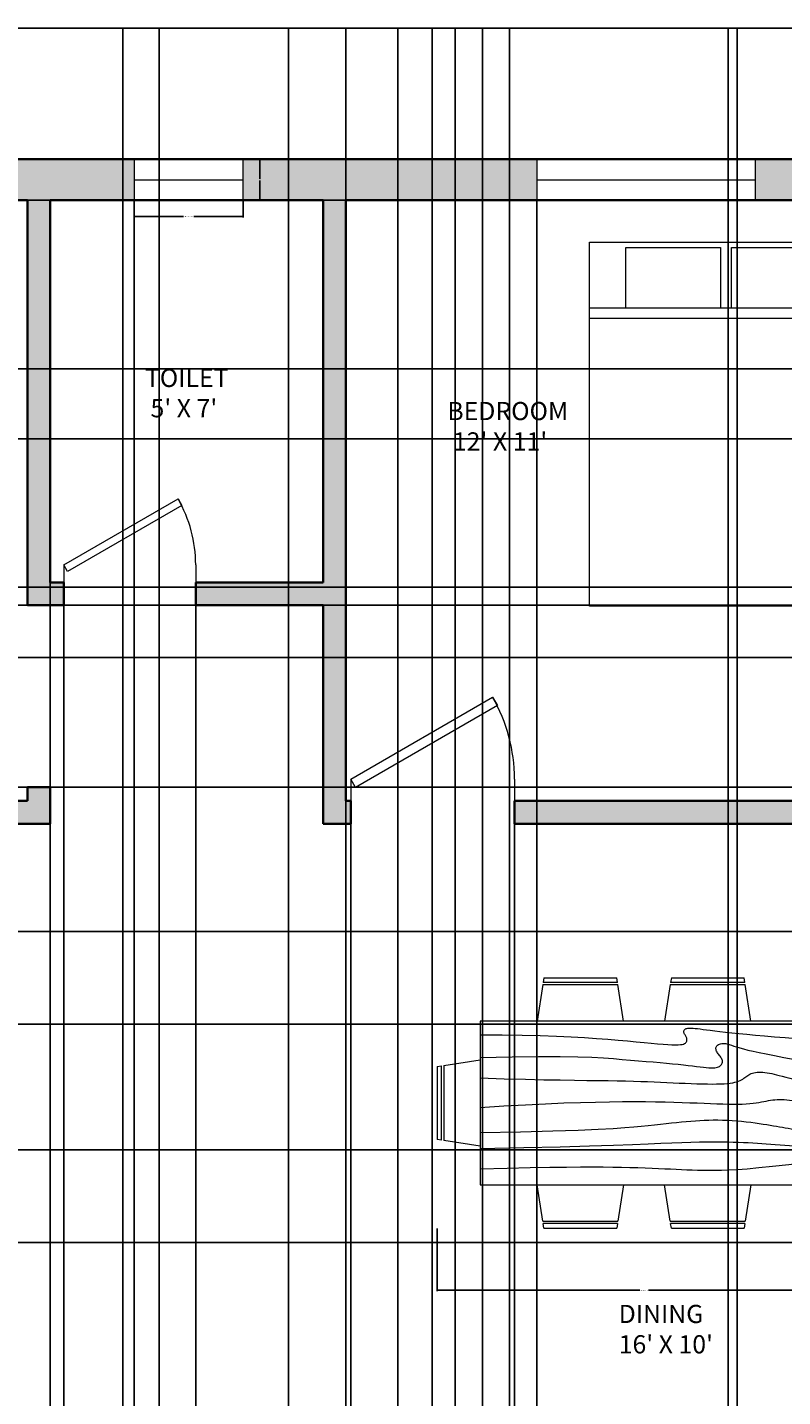
# Model space of a CAD drawing. Units: inches. Extents: x -28 to 649, y -11 to 509.
# Tile 4 of 7: x 180 to 346, y 208 to 509. Entities that reach past the tile are written whole.
import ezdxf

# ---------------------------------------------------------------- set-up
doc = ezdxf.new("R2010")
doc.units = ezdxf.units.IN
doc.header["$MEASUREMENT"] = 0
for name, color, linetype, lineweight in [('A-ANNO-DIMS', 2, 'Continuous', 18), ('A-AREA-IDEN', 18, 'Continuous', 18), ('A-WALL', 7, 'Continuous', 35), ('A-WALL-PATT', 251, 'Continuous', 13), ('doors', 40, 'Continuous', 20), ('furniture', 220, 'Continuous', 18), ('window', 30, 'Continuous', 18)]:
    doc.layers.add(name, color=color, linetype=linetype, lineweight=lineweight)
doc.styles.get("Standard").update_dxf_attribs({"font": 'arial.ttf'})
doc.dimstyles.get("Standard").update_dxf_attribs({"dimtxt": 0.18, "dimasz": 0.18, "dimexe": 0.18, "dimexo": 0.0625, "dimgap": 0.09, "dimtad": 0, "dimtih": 1, "dimtoh": 1, "dimdec": 4, "dimzin": 0, "dimdsep": 46, "dimtxsty": 'Standard', "dimcen": 0.09, "dimadec": 0, "dimazin": 0, "dimtfac": 1, "dimtdec": 4, "dimtofl": 0, "dimtmove": 0, "dimatfit": 3, "dimfxl": 1, "dimtolj": 1, "dimtzin": 0, "dimarcsym": 0})

# ---------------------------------------------------------------- blocks, each defined once
blk = doc.blocks.new('*U9')
for p, q in [((0, 0), (0, -100)), ((750, 0), (750, -100))]:
    blk.add_line(p, q)
blk.add_lwpolyline([(0, 0), (649.5, 375), (671.4, 337.1), (21.9, -37.9)], close=True)
blk.add_arc((0, 0), 750, 0, 30)
blk = doc.blocks.new('Dining Set - 36 x 72 in.')
for p, q in [((-22, 27.5), (-22.1562, 26.50042)), ((-22, 27.5), (-6, 27.5)), ((-5.8437, 26.49966), (-6, 27.5)), ((6, 27.5), (5.8438, 26.50042)), ((6, 27.5), (22, 27.5)), ((22.1563, 26.49966), (22, 27.5)), ((-22.2343, 26.00059), (-23.4847, 17.99762)), ((-22.2304, 26), (-5.7608, 26)), ((-5.8416, 26.5), (-22.1534, 26.5)), ((-4.5152, 17.99762), (-5.7655, 25.99926)), ((5.7657, 26.00059), (4.5153, 17.99762)), ((5.7696, 26), (22.2392, 26)), ((22.1584, 26.5), (5.8466, 26.5)), ((23.4848, 17.99762), (22.2345, 25.99926)), ((36, 18), (-36, 18)), ((-36, 18), (-36, -18)), ((36, -18), (36, 18)), ((-44.0006, 8.23428), (-35.9976, 9.48474)), ((44.0006, 8.23428), (35.9976, 9.48474)), ((-45.5, 8), (-44.5004, 8.15617)), ((-45.5, 8), (-45.5, -8)), ((-44.5, -8.15843), (-44.5, 8.15338)), ((-44, 8.23041), (-44, -8.23915)), ((44, 8.23041), (44, -8.23915)), ((44.5, -8.15843), (44.5, 8.15338)), ((45.5, 8), (44.5005, 8.15617)), ((45.5, 8), (45.5, -8)), ((-44.4997, -8.15631), (-45.5, -8)), ((-35.9976, -9.48476), (-43.9993, -8.2345)), ((35.9976, -9.48476), (43.9993, -8.2345)), ((44.4997, -8.15631), (45.5, -8)), ((-36, -18), (36, -18)), ((-22.2343, -26.0006), (-23.4847, -17.99762)), ((-4.5152, -17.99762), (-5.7655, -25.99928)), ((5.7657, -26.0006), (4.5153, -17.99762)), ((23.4848, -17.99762), (22.2345, -25.99928)), ((-22.2304, -26), (-5.7608, -26)), ((-22, -27.5), (-22.1562, -26.50044)), ((-5.8416, -26.5), (-22.1534, -26.5)), ((-5.8437, -26.49967), (-6, -27.5)), ((5.7696, -26), (22.2392, -26)), ((6, -27.5), (5.8438, -26.50044)), ((22.1584, -26.5), (5.8466, -26.5)), ((22.1563, -26.49967), (22, -27.5)), ((-22, -27.5), (-6, -27.5)), ((6, -27.5), (22, -27.5))]:
    blk.add_line(p, q)
for points in [[(-36, 15), (-31.1772, 14.97754), (-26.8079, 14.91406), (-22.8538, 14.81543), (-19.276, 14.6875), (-16.0362, 14.53613), (-13.0957, 14.36718), (-10.4159, 14.18652), (-7.9583, 14), (-5.6904, 13.81315), (-3.6035, 13.63021), (-1.6954, 13.45508), (0.0365, 13.29166), (1.5945, 13.14388), (2.9811, 13.01562), (4.1988, 12.9108), (5.25, 12.83333), (6.1393, 12.78613), (6.8802, 12.76823), (7.4883, 12.77767), (7.9792, 12.8125), (8.3685, 12.87077), (8.6719, 12.95052), (8.9049, 13.0498), (9.0833, 13.16666), (9.2205, 13.29899), (9.3216, 13.44401), (9.3895, 13.59879), (9.4271, 13.76041), (9.4373, 13.92594), (9.4232, 14.09245), (9.3875, 14.257), (9.3333, 14.41666), (9.2638, 14.56917), (9.1836, 14.71484), (9.0975, 14.85465), (9.0104, 14.98958), (8.9272, 15.1206), (8.8529, 15.2487), (8.7922, 15.37483), (8.75, 15.5), (8.7305, 15.62467), (8.7344, 15.74739), (8.7617, 15.86621), (8.8125, 15.97916), (8.8867, 16.08431), (8.9844, 16.17968), (9.1055, 16.26334), (9.25, 16.33333), (9.4189, 16.38802), (9.6172, 16.42708), (9.8506, 16.45052), (10.125, 16.45833), (10.4463, 16.45052), (10.8203, 16.42708), (11.2529, 16.38802), (11.75, 16.33333), (12.3184, 16.26318), (12.9694, 16.17838), (13.7151, 16.07991), (14.5677, 15.96875), (15.5395, 15.84586), (16.6426, 15.71224), (17.8893, 15.56884), (19.2917, 15.41666), (20.859, 15.25667), (22.5879, 15.08984), (24.4721, 14.91715), (26.5052, 14.73958), (28.6809, 14.5581), (30.9929, 14.3737), (33.4347, 14.18733), (36, 14)], [(-36, 10), (-28.9766, 10.14274), (-23.1725, 10.20442), (-18.4241, 10.19775), (-14.5677, 10.13541), (-11.4399, 10.03011), (-8.877, 9.89453), (-6.7154, 9.74137), (-4.7917, 9.58333), (-2.9698, 9.43082), (-1.2246, 9.28515), (0.4415, 9.14534), (2.026, 9.01041), (3.5266, 8.87939), (4.9408, 8.7513), (6.266, 8.62516), (7.5, 8.5), (8.6411, 8.37549), (9.6914, 8.2539), (10.6538, 8.13818), (11.5312, 8.03125), (12.3267, 7.93603), (13.043, 7.85547), (13.6831, 7.79248), (14.25, 7.75), (14.7471, 7.7303), (15.1797, 7.73307), (15.5537, 7.75732), (15.875, 7.80208), (16.1494, 7.86637), (16.3828, 7.94922), (16.5811, 8.04964), (16.75, 8.16666), (16.8944, 8.29915), (17.0143, 8.44531), (17.1089, 8.60319), (17.1771, 8.77083), (17.218, 8.94629), (17.2305, 9.1276), (17.2137, 9.31282), (17.1667, 9.5), (17.0895, 9.6875), (16.987, 9.875), (16.8649, 10.0625), (16.7292, 10.25), (16.5856, 10.4375), (16.4401, 10.625), (16.2985, 10.8125), (16.1667, 11), (16.05, 11.18733), (15.9518, 11.3737), (15.8752, 11.5581), (15.8229, 11.73958), (15.798, 11.91715), (15.8034, 12.08984), (15.842, 12.25667), (15.9167, 12.41666), (16.0295, 12.56836), (16.1784, 12.70833), (16.3605, 12.83268), (16.5729, 12.9375), (16.8127, 13.01888), (17.0768, 13.07291), (17.3625, 13.0957), (17.6667, 13.08333), (17.9894, 13.03312), (18.3418, 12.94726), (18.7382, 12.82918), (19.1927, 12.68229), (19.7195, 12.51001), (20.3327, 12.31575), (21.0465, 12.10294), (21.875, 11.875), (22.8357, 11.63354), (23.959, 11.37304), (25.2786, 11.08618), (26.8282, 10.76562), (28.6414, 10.40405), (30.752, 9.99414), (33.1936, 9.52856), (36, 9)], [(-36, 5.5), (-30.7157, 5.3348), (-26.069, 5.20963), (-21.9946, 5.11767), (-18.4271, 5.05208), (-15.3009, 5.00602), (-12.5508, 4.97265), (-10.1112, 4.94515), (-7.9167, 4.91666), (-5.909, 4.88167), (-4.0586, 4.83984), (-2.3429, 4.79215), (-0.7396, 4.73958), (0.7739, 4.6831), (2.22, 4.6237), (3.6213, 4.56233), (5, 4.5), (6.373, 4.43782), (7.7344, 4.3776), (9.0723, 4.32129), (10.375, 4.27083), (11.6309, 4.22819), (12.8281, 4.19531), (13.9551, 4.17415), (15, 4.16666), (15.954, 4.17448), (16.819, 4.19791), (17.6001, 4.23698), (18.3021, 4.29166), (18.9299, 4.36198), (19.4883, 4.44791), (19.9823, 4.54948), (20.4167, 4.66666), (20.7969, 4.79899), (21.1302, 4.94401), (21.4245, 5.09879), (21.6875, 5.26041), (21.9271, 5.42594), (22.1511, 5.59245), (22.3672, 5.757), (22.5834, 5.91666), (22.8065, 6.06868), (23.0404, 6.21093), (23.2879, 6.34147), (23.5521, 6.45833), (23.8358, 6.55957), (24.142, 6.64323), (24.4735, 6.70735), (24.8334, 6.75), (25.2235, 6.76969), (25.642, 6.76692), (26.0858, 6.74267), (26.5521, 6.69791), (27.0379, 6.63362), (27.5404, 6.55078), (28.0565, 6.45036), (28.5834, 6.33333), (29.1242, 6.19987), (29.7071, 6.04687), (30.3661, 5.87044), (31.1354, 5.66666), (32.0493, 5.43164), (33.142, 5.16146), (34.4475, 4.85221), (36, 4.5)], [(-36, -1), (-30.7915, -0.6591), (-26.0195, -0.38216), (-21.6519, -0.16284), (-17.6563, 0.00521), (-14.0005, 0.12833), (-10.6523, 0.21289), (-7.5796, 0.26522), (-4.75, 0.29166), (-2.134, 0.29793), (0.2878, 0.28711), (2.5317, 0.26163), (4.6146, 0.22396), (6.5529, 0.17651), (8.3633, 0.12174), (10.0623, 0.06209), (11.6667, 0), (13.1899, -0.06201), (14.6341, -0.1211), (15.9982, -0.17432), (17.2813, -0.21875), (18.4823, -0.25147), (19.6003, -0.26953), (20.6343, -0.27002), (21.5834, -0.25), (22.4481, -0.20768), (23.2357, -0.14584), (23.9549, -0.06836), (24.6146, 0.02083), (25.2235, 0.11784), (25.7904, 0.21875), (26.3241, 0.31966), (26.8334, 0.41666), (27.3265, 0.50618), (27.8099, 0.58593), (28.2894, 0.65397), (28.7709, 0.70833), (29.2601, 0.74707), (29.763, 0.76823), (30.2855, 0.76985), (30.8334, 0.75), (31.4088, 0.70784), (31.9994, 0.64713), (32.589, 0.57275), (33.1615, 0.48958), (33.7008, 0.4025), (34.1908, 0.3164), (34.6153, 0.23616), (34.9584, 0.16666), (35.2099, 0.11165), (35.3848, 0.07031), (35.504, 0.04069), (35.5886, 0.02083), (35.6594, 0.00879), (35.7377, 0.0026), (35.8442, 0.00032), (36, 0)], [(-36, -6.5), (-27.1843, -6.31267), (-20.084, -6.1263), (-14.469, -5.9419), (-10.1094, -5.76042), (-6.7752, -5.58285), (-4.2363, -5.41016), (-2.2629, -5.24333), (-0.625, -5.08334), (0.8708, -4.93099), (2.2715, -4.78646), (3.5872, -4.64974), (4.8281, -4.52084), (6.0046, -4.39974), (7.127, -4.28646), (8.2053, -4.18099), (9.25, -4.08334), (10.2705, -3.99382), (11.2734, -3.91407), (12.2647, -3.84603), (13.25, -3.79167), (14.2354, -3.75293), (15.2266, -3.73177), (16.2295, -3.73015), (17.25, -3.75), (18.2912, -3.79248), (19.3451, -3.85547), (20.4009, -3.93604), (21.4479, -4.03125), (22.4754, -4.13819), (23.4727, -4.25391), (24.4289, -4.37549), (25.3334, -4.5), (26.1785, -4.62492), (26.9694, -4.74935), (27.7145, -4.87281), (28.4219, -4.99479), (29.1, -5.11483), (29.7572, -5.23242), (30.4016, -5.34709), (31.0417, -5.45834), (31.6837, -5.56437), (32.3262, -5.65821), (32.9658, -5.73153), (33.599, -5.77604), (34.2224, -5.78345), (34.8327, -5.74545), (35.4264, -5.65373), (36, -5.5)], [(-36, -10), (-26.4022, -9.81299), (-18.4675, -9.62891), (-11.9839, -9.45069), (-6.7396, -9.28125), (-2.5226, -9.12354), (0.8789, -8.98047), (3.6769, -8.85498), (6.0833, -8.75), (8.2767, -8.66765), (10.3021, -8.60677), (12.1712, -8.56543), (13.8958, -8.54167), (15.4876, -8.53353), (16.9583, -8.53907), (18.3197, -8.55632), (19.5834, -8.58334), (20.7616, -8.61841), (21.8685, -8.66081), (22.9188, -8.71004), (23.9271, -8.76563), (24.9081, -8.82707), (25.8763, -8.89388), (26.8465, -8.96558), (27.8334, -9.04167), (28.8474, -9.12118), (29.8828, -9.20117), (30.93, -9.27824), (31.9792, -9.34896), (33.0205, -9.40991), (34.0443, -9.45768), (35.0407, -9.48885), (36, -9.5)], [(-36, -14.5), (-30.0881, -14.33513), (-25.0332, -14.21224), (-20.7312, -14.12647), (-17.0781, -14.07292), (-13.97, -14.04671), (-11.3027, -14.04297), (-8.9724, -14.05681), (-6.875, -14.08334), (-4.9224, -14.11833), (-3.0905, -14.16016), (-1.3709, -14.20785), (0.2448, -14.26042), (1.7647, -14.3169), (3.1973, -14.3763), (4.5507, -14.43767), (5.8333, -14.5), (7.0554, -14.5621), (8.235, -14.62175), (9.3922, -14.67652), (10.5469, -14.72396), (11.7192, -14.76164), (12.929, -14.78711), (14.1965, -14.79794), (15.5417, -14.79167), (16.9933, -14.76424), (18.6152, -14.70508), (20.4804, -14.60197), (22.6615, -14.44271), (25.2312, -14.21509), (28.2624, -13.9069), (31.8277, -13.50594), (36, -13)]]:
    blk.add_lwpolyline(points)
blk = doc.blocks.new('Bed - Queen')
for p, q in [((0, -80.00003), (0, 0)), ((0, 0), (59.99999, 0)), ((59.99999, 0), (59.99999, -80.00003)), ((7.99999, -1.2), (28.79998, -1.2)), ((7.99999, -14.4), (7.99999, -1.2)), ((28.79998, -1.2), (28.79998, -14.4)), ((31.19999, -1.2), (51.99999, -1.2)), ((31.19999, -14.4), (31.19999, -1.2)), ((51.99999, -1.2), (51.99999, -16.4)), ((0, -14.4), (44.8, -14.4)), ((59.99999, -29.6), (44.8, -14.4)), ((44.8, -14.4), (44.8, -29.6)), ((44.8, -16.8), (0, -16.8)), ((51.99999, -16.4), (46.79936, -16.4)), ((44.8, -29.6), (59.99999, -29.6)), ((59.99999, -80.00003), (0, -80.00003))]:
    blk.add_line(p, q)
blk = doc.blocks.new('WIN-48x9')
for p, q in [((9, 48), (0, 48)), ((0, 48), (0, 0)), ((4.5, 0), (4.5, 48)), ((9, 0), (9, 48)), ((0, 0), (9, 0)), ((0, 0), (4.5, 0))]:
    blk.add_line(p, q)
blk = doc.blocks.new('WIN-24x9')
for p, q in [((0, 9), (0, 0)), ((24, 9), (0, 9)), ((0, 9), (0, 4.5)), ((24, 0), (24, 9)), ((0, 4.5), (24, 4.5)), ((0, 0), (24, 0))]:
    blk.add_line(p, q)
blk = doc.blocks.new('*D18')
at = {"layer": 'A-ANNO-DIMS', "color": 0, "lineweight": -2, "transparency": 16777216}
for p, q in [((203.91, 470.88), (203.91, 467.16)), ((227.91, 470.88), (227.91, 467.16)), ((204.09, 467.34), (214.79, 467.34)), ((227.73, 467.34), (217.03, 467.34))]:
    blk.add_line(p, q, dxfattribs=at)
at = {"layer": 'A-ANNO-DIMS', "color": 0, "transparency": 16777216}
for points in [[(204.09, 467.37), (204.09, 467.31), (203.91, 467.34)], [(227.73, 467.37), (227.73, 467.31), (227.91, 467.34)]]:
    blk.add_solid(points, dxfattribs=at)
at = {"layer": 'Defpoints', "color": 0, "transparency": 16777216}
for p in [(203.91, 470.94), (227.91, 470.94), (227.91, 467.34)]:
    blk.add_point(p, dxfattribs=at)
at = {"layer": 'A-ANNO-DIMS', "color": 0, "transparency": 16777216, "insert": (215.91, 467.34), "char_height": 0.18, "attachment_point": 5}
blk.add_mtext('\\A1;WINDOW 24 TYP.', dxfattribs=at)
blk = doc.blocks.new('*D19')
at = {"layer": 'A-ANNO-DIMS', "color": 0, "lineweight": -2, "transparency": 16777216}
for p, q in [((227.97, 479.94), (231.69, 479.94)), ((231.51, 479.76), (231.51, 475.62)), ((231.51, 471.12), (231.51, 475.26)), ((227.97, 470.94), (231.69, 470.94))]:
    blk.add_line(p, q, dxfattribs=at)
at = {"layer": 'A-ANNO-DIMS', "color": 0, "transparency": 16777216}
for points in [[(231.48, 479.76), (231.54, 479.76), (231.51, 479.94)], [(231.48, 471.12), (231.54, 471.12), (231.51, 470.94)]]:
    blk.add_solid(points, dxfattribs=at)
at = {"layer": 'Defpoints', "color": 0, "transparency": 16777216}
for p in [(227.91, 479.94), (231.51, 479.94), (227.91, 470.94)]:
    blk.add_point(p, dxfattribs=at)
at = {"layer": 'A-ANNO-DIMS', "color": 0, "transparency": 16777216, "insert": (231.51, 475.44), "char_height": 0.18, "attachment_point": 5}
blk.add_mtext('\\A1;9 TYP.', dxfattribs=at)
blk = doc.blocks.new('*D28')
at = {"layer": 'A-ANNO-DIMS', "color": 0, "lineweight": -2, "transparency": 16777216}
for p, q in [((270.49, 245), (270.49, 231.23)), ((361.49, 245), (361.49, 231.23)), ((270.67, 231.41), (315.04, 231.41)), ((361.31, 231.41), (316.94, 231.41))]:
    blk.add_line(p, q, dxfattribs=at)
at = {"layer": 'A-ANNO-DIMS', "color": 0, "transparency": 16777216}
for points in [[(270.67, 231.44), (270.67, 231.38), (270.49, 231.41)], [(361.31, 231.44), (361.31, 231.38), (361.49, 231.41)]]:
    blk.add_solid(points, dxfattribs=at)
at = {"layer": 'Defpoints', "color": 0, "transparency": 16777216}
for p in [(270.49, 245.06), (361.49, 245.06), (361.49, 231.41)]:
    blk.add_point(p, dxfattribs=at)
at = {"layer": 'A-ANNO-DIMS', "color": 0, "transparency": 16777216, "insert": (315.99, 231.41), "char_height": 0.18, "attachment_point": 5}
blk.add_mtext('\\A1;DINING SET 91', dxfattribs=at)
blk = doc.blocks.new('*D30')
at = {"layer": 'A-ANNO-DIMS', "color": 0, "lineweight": -2, "transparency": 16777216}
for p, q in [((27.45, 480), (27.45, 508.92)), ((27.63, 508.74), (315.16, 508.74)), ((603.27, 508.74), (315.74, 508.74)), ((603.45, 480), (603.45, 508.92))]:
    blk.add_line(p, q, dxfattribs=at)
at = {"layer": 'A-ANNO-DIMS', "color": 0, "transparency": 16777216}
for points in [[(27.63, 508.77), (27.63, 508.71), (27.45, 508.74)], [(603.27, 508.77), (603.27, 508.71), (603.45, 508.74)]]:
    blk.add_solid(points, dxfattribs=at)
at = {"layer": 'Defpoints', "color": 0, "transparency": 16777216}
for p in [(603.45, 508.74), (27.45, 479.94), (603.45, 479.94)]:
    blk.add_point(p, dxfattribs=at)
at = {"layer": 'A-ANNO-DIMS', "color": 0, "transparency": 16777216, "insert": (315.45, 508.74), "char_height": 0.18, "attachment_point": 5}
blk.add_mtext('\\A1;576', dxfattribs=at)
blk = doc.blocks.new('*D31')
at = {"layer": 'A-ANNO-DIMS', "color": 0, "lineweight": -2, "transparency": 16777216}
for p, q in [((603.51, 479.94), (632.43, 479.94)), ((632.25, 479.76), (632.25, 249.12)), ((632.25, 18.12), (632.25, 248.76)), ((346.51, 17.94), (632.43, 17.94))]:
    blk.add_line(p, q, dxfattribs=at)
at = {"layer": 'A-ANNO-DIMS', "color": 0, "transparency": 16777216}
for points in [[(632.22, 479.76), (632.28, 479.76), (632.25, 479.94)], [(632.22, 18.12), (632.28, 18.12), (632.25, 17.94)]]:
    blk.add_solid(points, dxfattribs=at)
at = {"layer": 'Defpoints', "color": 0, "transparency": 16777216}
for p in [(603.45, 479.94), (632.25, 479.94), (346.45, 17.94)]:
    blk.add_point(p, dxfattribs=at)
at = {"layer": 'A-ANNO-DIMS', "color": 0, "transparency": 16777216, "insert": (632.25, 248.94), "char_height": 0.18, "attachment_point": 5}
blk.add_mtext('\\A1;462', dxfattribs=at)
blk = doc.blocks.new('*D34')
at = {"layer": 'A-ANNO-DIMS', "color": 0, "lineweight": -2, "transparency": 16777216}
for p, q in [((280.45, 48), (280.45, 508.92)), ((280.63, 508.74), (308.23, 508.74)), ((336.27, 508.74), (308.67, 508.74)), ((336.45, 48), (336.45, 508.92))]:
    blk.add_line(p, q, dxfattribs=at)
at = {"layer": 'A-ANNO-DIMS', "color": 0, "transparency": 16777216}
for points in [[(280.63, 508.77), (280.63, 508.71), (280.45, 508.74)], [(336.27, 508.77), (336.27, 508.71), (336.45, 508.74)]]:
    blk.add_solid(points, dxfattribs=at)
at = {"layer": 'Defpoints', "color": 0, "transparency": 16777216}
for p in [(336.45, 508.74), (280.45, 47.94), (336.45, 47.94)]:
    blk.add_point(p, dxfattribs=at)
at = {"layer": 'A-ANNO-DIMS', "color": 0, "transparency": 16777216, "insert": (308.45, 508.74), "char_height": 0.18, "attachment_point": 5}
blk.add_mtext('\\A1;56', dxfattribs=at)
blk = doc.blocks.new('*D45')
at = {"layer": 'A-ANNO-DIMS', "color": 0, "lineweight": -2, "transparency": 16777216}
for p, q in [((185.45, 470.88), (185.45, -11.04)), ((203.91, 470.88), (203.91, -11.04)), ((185.63, -10.86), (194.29, -10.86)), ((203.73, -10.86), (195.07, -10.86))]:
    blk.add_line(p, q, dxfattribs=at)
at = {"layer": 'A-ANNO-DIMS', "color": 0, "transparency": 16777216}
for points in [[(185.63, -10.83), (185.63, -10.89), (185.45, -10.86)], [(203.73, -10.83), (203.73, -10.89), (203.91, -10.86)]]:
    blk.add_solid(points, dxfattribs=at)
at = {"layer": 'Defpoints', "color": 0, "transparency": 16777216}
for p in [(185.45, 470.94), (203.91, 470.94), (203.91, -10.86)]:
    blk.add_point(p, dxfattribs=at)
at = {"layer": 'A-ANNO-DIMS', "color": 0, "transparency": 16777216, "insert": (194.68, -10.86), "char_height": 0.18, "attachment_point": 5}
blk.add_mtext('\\A1;18.46', dxfattribs=at)
blk = doc.blocks.new('*D46')
at = {"layer": 'A-ANNO-DIMS', "color": 0, "lineweight": -2, "transparency": 16777216}
for p, q in [((250.45, 470.88), (250.45, -11.04)), ((292.46, 470.88), (292.46, -11.04)), ((250.63, -10.86), (271.08, -10.86)), ((292.28, -10.86), (271.83, -10.86))]:
    blk.add_line(p, q, dxfattribs=at)
at = {"layer": 'A-ANNO-DIMS', "color": 0, "transparency": 16777216}
for points in [[(250.63, -10.83), (250.63, -10.89), (250.45, -10.86)], [(292.28, -10.83), (292.28, -10.89), (292.46, -10.86)]]:
    blk.add_solid(points, dxfattribs=at)
at = {"layer": 'Defpoints', "color": 0, "transparency": 16777216}
for p in [(250.45, 470.94), (292.46, 470.94), (292.46, -10.86)]:
    blk.add_point(p, dxfattribs=at)
at = {"layer": 'A-ANNO-DIMS', "color": 0, "transparency": 16777216, "insert": (271.45, -10.86), "char_height": 0.18, "attachment_point": 5}
blk.add_mtext('\\A1;42.01', dxfattribs=at)
blk = doc.blocks.new('*D49')
at = {"layer": 'A-ANNO-DIMS', "color": 0, "lineweight": -2, "transparency": 16777216}
for p, q in [((36.51, 470.94), (632.43, 470.94)), ((632.25, 470.76), (632.25, 452.59)), ((632.25, 434.06), (632.25, 452.23)), ((36.51, 433.88), (632.43, 433.88))]:
    blk.add_line(p, q, dxfattribs=at)
at = {"layer": 'A-ANNO-DIMS', "color": 0, "transparency": 16777216}
for points in [[(632.22, 470.76), (632.28, 470.76), (632.25, 470.94)], [(632.22, 434.06), (632.28, 434.06), (632.25, 433.88)]]:
    blk.add_solid(points, dxfattribs=at)
at = {"layer": 'Defpoints', "color": 0, "transparency": 16777216}
for p in [(36.45, 470.94), (36.45, 433.88), (632.25, 433.88)]:
    blk.add_point(p, dxfattribs=at)
at = {"layer": 'A-ANNO-DIMS', "color": 0, "transparency": 16777216, "insert": (632.25, 452.41), "char_height": 0.18, "attachment_point": 5}
blk.add_mtext('\\A1;37.055', dxfattribs=at)
blk = doc.blocks.new('*D50')
at = {"layer": 'A-ANNO-DIMS', "color": 0, "lineweight": -2, "transparency": 16777216}
for p, q in [((594.39, 470.94), (-1.53, 470.94)), ((-1.35, 470.76), (-1.35, 444.89)), ((-1.35, 418.66), (-1.35, 444.53)), ((594.39, 418.48), (-1.53, 418.48))]:
    blk.add_line(p, q, dxfattribs=at)
at = {"layer": 'A-ANNO-DIMS', "color": 0, "transparency": 16777216}
for points in [[(-1.38, 470.76), (-1.32, 470.76), (-1.35, 470.94)], [(-1.38, 418.66), (-1.32, 418.66), (-1.35, 418.48)]]:
    blk.add_solid(points, dxfattribs=at)
at = {"layer": 'Defpoints', "color": 0, "transparency": 16777216}
for p in [(594.45, 470.94), (-1.35, 418.48), (594.45, 418.48)]:
    blk.add_point(p, dxfattribs=at)
at = {"layer": 'A-ANNO-DIMS', "color": 0, "transparency": 16777216, "insert": (-1.35, 444.71), "char_height": 0.18, "attachment_point": 5}
blk.add_mtext('\\A1;52.46', dxfattribs=at)
blk = doc.blocks.new('*D51')
at = {"layer": 'A-ANNO-DIMS', "color": 0, "lineweight": -2, "transparency": 16777216}
for p, q in [((594.39, 370.48), (-1.53, 370.48)), ((-1.35, 370.3), (-1.35, 340.55)), ((-1.35, 310.43), (-1.35, 340.19)), ((594.39, 310.25), (-1.53, 310.25))]:
    blk.add_line(p, q, dxfattribs=at)
at = {"layer": 'A-ANNO-DIMS', "color": 0, "transparency": 16777216}
for points in [[(-1.38, 370.3), (-1.32, 370.3), (-1.35, 370.48)], [(-1.38, 310.43), (-1.32, 310.43), (-1.35, 310.25)]]:
    blk.add_solid(points, dxfattribs=at)
at = {"layer": 'Defpoints', "color": 0, "transparency": 16777216}
for p in [(-1.35, 370.48), (594.45, 370.48), (594.45, 310.25)]:
    blk.add_point(p, dxfattribs=at)
at = {"layer": 'A-ANNO-DIMS', "color": 0, "transparency": 16777216, "insert": (-1.35, 340.37), "char_height": 0.18, "attachment_point": 5}
blk.add_mtext('\\A1;60.23', dxfattribs=at)
blk = doc.blocks.new('*D52')
at = {"layer": 'A-ANNO-DIMS', "color": 0, "lineweight": -2, "transparency": 16777216}
for p, q in [((594.39, 262.25), (-1.53, 262.25)), ((-1.35, 262.07), (-1.35, 206.61)), ((-1.35, 150.79), (-1.35, 206.25)), ((594.39, 150.61), (-1.53, 150.61))]:
    blk.add_line(p, q, dxfattribs=at)
at = {"layer": 'A-ANNO-DIMS', "color": 0, "transparency": 16777216}
for points in [[(-1.38, 262.07), (-1.32, 262.07), (-1.35, 262.25)], [(-1.38, 150.79), (-1.32, 150.79), (-1.35, 150.61)]]:
    blk.add_solid(points, dxfattribs=at)
at = {"layer": 'Defpoints', "color": 0, "transparency": 16777216}
for p in [(-1.35, 262.25), (594.45, 262.25), (594.45, 150.61)]:
    blk.add_point(p, dxfattribs=at)
at = {"layer": 'A-ANNO-DIMS', "color": 0, "transparency": 16777216, "insert": (-1.35, 206.43), "char_height": 0.18, "attachment_point": 5}
blk.add_mtext('\\A1;111.64', dxfattribs=at)
blk = doc.blocks.new('*D53')
at = {"layer": 'A-ANNO-DIMS', "color": 0, "lineweight": -2, "transparency": 16777216}
for p, q in [((36.51, 241.9), (632.43, 241.9)), ((632.25, 241.72), (632.25, 191.76)), ((632.25, 141.44), (632.25, 191.39)), ((36.51, 141.26), (632.43, 141.26))]:
    blk.add_line(p, q, dxfattribs=at)
at = {"layer": 'A-ANNO-DIMS', "color": 0, "transparency": 16777216}
for points in [[(632.22, 241.72), (632.28, 241.72), (632.25, 241.9)], [(632.22, 141.44), (632.28, 141.44), (632.25, 141.26)]]:
    blk.add_solid(points, dxfattribs=at)
at = {"layer": 'Defpoints', "color": 0, "transparency": 16777216}
for p in [(36.45, 241.9), (632.25, 241.9), (36.45, 141.26)]:
    blk.add_point(p, dxfattribs=at)
at = {"layer": 'A-ANNO-DIMS', "color": 0, "transparency": 16777216, "insert": (632.25, 191.58), "char_height": 0.18, "attachment_point": 5}
blk.add_mtext('\\A1;100.64', dxfattribs=at)
blk = doc.blocks.new('*D54')
at = {"layer": 'A-ANNO-DIMS', "color": 0, "lineweight": -2, "transparency": 16777216}
for p, q in [((36.51, 385.88), (632.43, 385.88)), ((632.25, 385.7), (632.25, 338.07)), ((632.25, 290.08), (632.25, 337.71)), ((36.51, 289.9), (632.43, 289.9))]:
    blk.add_line(p, q, dxfattribs=at)
at = {"layer": 'A-ANNO-DIMS', "color": 0, "transparency": 16777216}
for points in [[(632.22, 385.7), (632.28, 385.7), (632.25, 385.88)], [(632.22, 290.08), (632.28, 290.08), (632.25, 289.9)]]:
    blk.add_solid(points, dxfattribs=at)
at = {"layer": 'Defpoints', "color": 0, "transparency": 16777216}
for p in [(36.45, 385.88), (632.25, 385.88), (36.45, 289.9)]:
    blk.add_point(p, dxfattribs=at)
at = {"layer": 'A-ANNO-DIMS', "color": 0, "transparency": 16777216, "insert": (632.25, 337.89), "char_height": 0.18, "attachment_point": 5}
blk.add_mtext('\\A1;95.99', dxfattribs=at)
blk = doc.blocks.new('*D56')
at = {"layer": 'A-ANNO-DIMS', "color": 0, "lineweight": -2, "transparency": 16777216}
for p, q in [((286.45, 89), (286.45, 508.92)), ((286.63, 508.74), (310.23, 508.74)), ((334.27, 508.74), (310.67, 508.74)), ((334.45, 89), (334.45, 508.92))]:
    blk.add_line(p, q, dxfattribs=at)
at = {"layer": 'A-ANNO-DIMS', "color": 0, "transparency": 16777216}
for points in [[(286.63, 508.77), (286.63, 508.71), (286.45, 508.74)], [(334.27, 508.77), (334.27, 508.71), (334.45, 508.74)]]:
    blk.add_solid(points, dxfattribs=at)
at = {"layer": 'Defpoints', "color": 0, "transparency": 16777216}
for p in [(334.45, 508.74), (286.45, 88.94), (334.45, 88.94)]:
    blk.add_point(p, dxfattribs=at)
at = {"layer": 'A-ANNO-DIMS', "color": 0, "transparency": 16777216, "insert": (310.45, 508.74), "char_height": 0.18, "attachment_point": 5}
blk.add_mtext('\\A1;48', dxfattribs=at)
blk = doc.blocks.new('*D57')
at = {"layer": 'A-ANNO-DIMS', "color": 0, "lineweight": -2, "transparency": 16777216}
for p, q in [((165.45, 190), (165.45, 508.92)), ((165.63, 508.74), (183.23, 508.74)), ((201.27, 508.74), (183.67, 508.74)), ((201.45, 190), (201.45, 508.92))]:
    blk.add_line(p, q, dxfattribs=at)
at = {"layer": 'A-ANNO-DIMS', "color": 0, "transparency": 16777216}
for points in [[(165.63, 508.77), (165.63, 508.71), (165.45, 508.74)], [(201.27, 508.77), (201.27, 508.71), (201.45, 508.74)]]:
    blk.add_solid(points, dxfattribs=at)
at = {"layer": 'Defpoints', "color": 0, "transparency": 16777216}
for p in [(201.45, 508.74), (165.45, 189.94), (201.45, 189.94)]:
    blk.add_point(p, dxfattribs=at)
at = {"layer": 'A-ANNO-DIMS', "color": 0, "transparency": 16777216, "insert": (183.45, 508.74), "char_height": 0.18, "attachment_point": 5}
blk.add_mtext('\\A1;36', dxfattribs=at)
blk = doc.blocks.new('*D62')
at = {"layer": 'A-ANNO-DIMS', "color": 0, "lineweight": -2, "transparency": 16777216}
for p, q in [((188.45, 381.88), (188.45, -11.04)), ((217.45, 381.88), (217.45, -11.04)), ((188.63, -10.86), (202.73, -10.86)), ((217.27, -10.86), (203.17, -10.86))]:
    blk.add_line(p, q, dxfattribs=at)
at = {"layer": 'A-ANNO-DIMS', "color": 0, "transparency": 16777216}
for points in [[(188.63, -10.83), (188.63, -10.89), (188.45, -10.86)], [(217.27, -10.83), (217.27, -10.89), (217.45, -10.86)]]:
    blk.add_solid(points, dxfattribs=at)
at = {"layer": 'Defpoints', "color": 0, "transparency": 16777216}
for p in [(188.45, 381.94), (217.45, 381.94), (217.45, -10.86)]:
    blk.add_point(p, dxfattribs=at)
at = {"layer": 'A-ANNO-DIMS', "color": 0, "transparency": 16777216, "insert": (202.95, -10.86), "char_height": 0.18, "attachment_point": 5}
blk.add_mtext('\\A1;29', dxfattribs=at)
blk = doc.blocks.new('*D64')
at = {"layer": 'A-ANNO-DIMS', "color": 0, "lineweight": -2, "transparency": 16777216}
for p, q in [((251.52, 333.88), (251.52, -11.04)), ((287.52, 333.88), (287.52, -11.04)), ((251.7, -10.86), (269.3, -10.86)), ((287.34, -10.86), (269.74, -10.86))]:
    blk.add_line(p, q, dxfattribs=at)
at = {"layer": 'A-ANNO-DIMS', "color": 0, "transparency": 16777216}
for points in [[(251.7, -10.83), (251.7, -10.89), (251.52, -10.86)], [(287.34, -10.83), (287.34, -10.89), (287.52, -10.86)]]:
    blk.add_solid(points, dxfattribs=at)
at = {"layer": 'Defpoints', "color": 0, "transparency": 16777216}
for p in [(251.52, 333.94), (287.52, 333.94), (287.52, -10.86)]:
    blk.add_point(p, dxfattribs=at)
at = {"layer": 'A-ANNO-DIMS', "color": 0, "transparency": 16777216, "insert": (269.52, -10.86), "char_height": 0.18, "attachment_point": 5}
blk.add_mtext('\\A1;36', dxfattribs=at)
blk = doc.blocks.new('*D65')
at = {"layer": 'A-ANNO-DIMS', "color": 0, "lineweight": -2, "transparency": 16777216}
for p, q in [((185.51, 381.94), (632.43, 381.94)), ((632.25, 381.76), (632.25, 362.12)), ((632.25, 342.12), (632.25, 361.76)), ((185.51, 341.94), (632.43, 341.94))]:
    blk.add_line(p, q, dxfattribs=at)
at = {"layer": 'A-ANNO-DIMS', "color": 0, "transparency": 16777216}
for points in [[(632.22, 381.76), (632.28, 381.76), (632.25, 381.94)], [(632.22, 342.12), (632.28, 342.12), (632.25, 341.94)]]:
    blk.add_solid(points, dxfattribs=at)
at = {"layer": 'Defpoints', "color": 0, "transparency": 16777216}
for p in [(185.45, 381.94), (632.25, 381.94), (185.45, 341.94)]:
    blk.add_point(p, dxfattribs=at)
at = {"layer": 'A-ANNO-DIMS', "color": 0, "transparency": 16777216, "insert": (632.25, 361.94), "char_height": 0.18, "attachment_point": 5}
blk.add_mtext('\\A1;40', dxfattribs=at)
blk = doc.blocks.new('*D66')
at = {"layer": 'A-ANNO-DIMS', "color": 0, "lineweight": -2, "transparency": 16777216}
for p, q in [((447.05, 381.94), (-1.53, 381.94)), ((-1.35, 381.76), (-1.35, 362.12)), ((-1.35, 342.12), (-1.35, 361.76)), ((447.39, 341.94), (-1.53, 341.94))]:
    blk.add_line(p, q, dxfattribs=at)
at = {"layer": 'A-ANNO-DIMS', "color": 0, "transparency": 16777216}
for points in [[(-1.38, 381.76), (-1.32, 381.76), (-1.35, 381.94)], [(-1.38, 342.12), (-1.32, 342.12), (-1.35, 341.94)]]:
    blk.add_solid(points, dxfattribs=at)
at = {"layer": 'Defpoints', "color": 0, "transparency": 16777216}
for p in [(-1.35, 381.94), (447.12, 381.94), (447.45, 341.94)]:
    blk.add_point(p, dxfattribs=at)
at = {"layer": 'A-ANNO-DIMS', "color": 0, "transparency": 16777216, "insert": (-1.35, 361.94), "char_height": 0.18, "attachment_point": 5}
blk.add_mtext('\\A1;40', dxfattribs=at)
blk = doc.blocks.new('*D67')
at = {"layer": 'A-ANNO-DIMS', "color": 0, "lineweight": -2, "transparency": 16777216}
for p, q in [((250.45, 471), (250.45, 508.92)), ((250.63, 508.74), (316.17, 508.74)), ((382.27, 508.74), (316.73, 508.74)), ((382.45, 471), (382.45, 508.92))]:
    blk.add_line(p, q, dxfattribs=at)
at = {"layer": 'A-ANNO-DIMS', "color": 0, "transparency": 16777216}
for points in [[(250.63, 508.77), (250.63, 508.71), (250.45, 508.74)], [(382.27, 508.77), (382.27, 508.71), (382.45, 508.74)]]:
    blk.add_solid(points, dxfattribs=at)
at = {"layer": 'Defpoints', "color": 0, "transparency": 16777216}
for p in [(382.45, 508.74), (250.45, 470.94), (382.45, 470.94)]:
    blk.add_point(p, dxfattribs=at)
at = {"layer": 'A-ANNO-DIMS', "color": 0, "transparency": 16777216, "insert": (316.45, 508.74), "char_height": 0.18, "attachment_point": 5}
blk.add_mtext('\\A1;132', dxfattribs=at)
blk = doc.blocks.new('*D74')
at = {"layer": 'A-ANNO-DIMS', "color": 0, "lineweight": -2, "transparency": 16777216}
for p, q in [((237.88, 89), (237.88, 508.92)), ((238.06, 508.74), (249.66, 508.74)), ((261.7, 508.74), (250.1, 508.74)), ((261.88, 89), (261.88, 508.92))]:
    blk.add_line(p, q, dxfattribs=at)
at = {"layer": 'A-ANNO-DIMS', "color": 0, "transparency": 16777216}
for points in [[(238.06, 508.77), (238.06, 508.71), (237.88, 508.74)], [(261.7, 508.77), (261.7, 508.71), (261.88, 508.74)]]:
    blk.add_solid(points, dxfattribs=at)
at = {"layer": 'Defpoints', "color": 0, "transparency": 16777216}
for p in [(261.88, 508.74), (237.88, 88.94), (261.88, 88.94)]:
    blk.add_point(p, dxfattribs=at)
at = {"layer": 'A-ANNO-DIMS', "color": 0, "transparency": 16777216, "insert": (249.88, 508.74), "char_height": 0.18, "attachment_point": 5}
blk.add_mtext('\\A1;24', dxfattribs=at)
blk = doc.blocks.new('*D75')
at = {"layer": 'A-ANNO-DIMS', "color": 0, "lineweight": -2, "transparency": 16777216}
for p, q in [((209.45, 89), (209.45, 508.92)), ((209.63, 508.74), (223.27, 508.74)), ((237.7, 508.74), (224.06, 508.74)), ((237.88, 89), (237.88, 508.92))]:
    blk.add_line(p, q, dxfattribs=at)
at = {"layer": 'A-ANNO-DIMS', "color": 0, "transparency": 16777216}
for points in [[(209.63, 508.77), (209.63, 508.71), (209.45, 508.74)], [(237.7, 508.77), (237.7, 508.71), (237.88, 508.74)]]:
    blk.add_solid(points, dxfattribs=at)
at = {"layer": 'Defpoints', "color": 0, "transparency": 16777216}
for p in [(237.88, 508.74), (209.45, 88.94), (237.88, 88.94)]:
    blk.add_point(p, dxfattribs=at)
at = {"layer": 'A-ANNO-DIMS', "color": 0, "transparency": 16777216, "insert": (223.66, 508.74), "char_height": 0.18, "attachment_point": 5}
blk.add_mtext('\\A1;28.43', dxfattribs=at)
blk = doc.blocks.new('*D76')
at = {"layer": 'A-ANNO-DIMS', "color": 0, "lineweight": -2, "transparency": 16777216}
for p, q in [((269.45, 185), (269.45, 508.92)), ((269.63, 508.74), (271.8, 508.74)), ((274.27, 508.74), (272.1, 508.74)), ((274.45, 190), (274.45, 508.92))]:
    blk.add_line(p, q, dxfattribs=at)
at = {"layer": 'A-ANNO-DIMS', "color": 0, "transparency": 16777216}
for points in [[(269.63, 508.77), (269.63, 508.71), (269.45, 508.74)], [(274.27, 508.77), (274.27, 508.71), (274.45, 508.74)]]:
    blk.add_solid(points, dxfattribs=at)
at = {"layer": 'Defpoints', "color": 0, "transparency": 16777216}
for p in [(274.45, 508.74), (274.45, 189.94), (269.45, 184.94)]:
    blk.add_point(p, dxfattribs=at)
at = {"layer": 'A-ANNO-DIMS', "color": 0, "transparency": 16777216, "insert": (271.95, 508.74), "char_height": 0.18, "attachment_point": 5}
blk.add_mtext('\\A1;5', dxfattribs=at)

msp = doc.modelspace()

# ---------------------------------------------------------------- hatches: boundary and pattern name
at = {"layer": 'A-WALL-PATT'}
h = msp.add_hatch(color=256, dxfattribs=at)
h.dxf.hatch_style = 1
h.paths.add_polyline_path([(36.4499, 184.9382), (165.4499, 184.9382), (165.4499, 189.9382), (36.4499, 189.9382), (36.4499, 241.898), (27.4499, 241.898), (27.4499, 141.2558), (36.4499, 141.2558)])
h.paths.add_polyline_path([(36.4499, 385.8835), (27.4499, 385.8835), (27.4499, 289.898), (36.4499, 289.898)])
h.paths.add_polyline_path([(185.4499, 341.9382), (180.4499, 341.9382), (180.4499, 338.9382), (36.4499, 338.9382), (36.4499, 333.9382), (185.4499, 333.9382)])
h.paths.add_polyline_path([(36.4499, 470.9382), (79.2168, 470.9382), (79.2168, 479.9382), (27.4499, 479.9382), (27.4499, 433.8835), (36.4499, 433.8835)])
h.paths.add_polyline_path([(185.4499, 470.9382), (203.9104, 470.9382), (203.9104, 479.9382), (127.2168, 479.9382), (127.2168, 470.9382), (180.4499, 470.9382), (180.4499, 381.9382), (188.4499, 381.9382), (188.4499, 386.9382), (185.4499, 386.9382)])
h.paths.add_polyline_path([(292.4601, 479.9382), (227.9104, 479.9382), (227.9104, 470.9382), (245.4499, 470.9382), (245.4499, 386.9382), (217.4499, 386.9382), (217.4499, 381.9382), (245.4499, 381.9382), (245.4499, 338.9382), (245.4499, 333.9382), (251.5222, 333.9382), (251.5222, 338.9382), (250.4499, 338.9382), (250.4499, 470.9382), (292.4601, 470.9382)])
h.paths.add_polyline_path([(410.9121, 479.9382), (340.4601, 479.9382), (340.4601, 470.9382), (382.4499, 470.9382), (382.4499, 338.9382), (287.5222, 338.9382), (287.5222, 333.9382), (387.4499, 333.9382), (387.4499, 381.9382), (415.4499, 381.9382), (415.4499, 386.9382), (387.4499, 386.9382), (387.4499, 470.9382), (410.9121, 470.9382)])
h.paths.add_polyline_path([(497.0961, 479.9382), (434.9121, 479.9382), (434.9121, 470.9382), (447.4499, 470.9382), (447.4499, 386.9382), (444.4499, 386.9382), (444.4499, 381.9382), (452.4499, 381.9382), (452.4499, 470.9382), (497.0961, 470.9382)])
h.paths.add_polyline_path([(603.4499, 479.9382), (545.0961, 479.9382), (545.0961, 470.9382), (594.4499, 470.9382), (594.4499, 418.4819), (603.4499, 418.4819)])
h.paths.add_polyline_path([(603.4499, 370.4819), (594.4499, 370.4819), (594.4499, 338.9382), (452.4499, 338.9382), (452.4499, 341.9382), (447.4499, 341.9382), (447.4499, 338.9382), (447.4499, 333.9382), (594.4499, 333.9382), (594.4499, 310.2528), (603.4499, 310.2528)])
h.paths.add_polyline_path([(603.4499, 262.2528), (594.4499, 262.2528), (594.4499, 205.9382), (515.4499, 205.9382), (515.4499, 200.9382), (594.4499, 200.9382), (594.4499, 150.6102), (603.4499, 150.6102)])

# ---------------------------------------------------------------- linework, layer by layer
at = {"layer": 'A-WALL'}
for p, q in [((36.4499, 470.9382), (180.4499, 470.9382)), ((180.4499, 381.9382), (180.4499, 470.9382)), ((185.4499, 470.9382), (245.4499, 470.9382)), ((185.4499, 386.9382), (185.4499, 470.9382)), ((245.4499, 386.9382), (245.4499, 470.9382)), ((250.4499, 470.9382), (382.4499, 470.9382)), ((250.4499, 338.9382), (250.4499, 470.9382)), ((185.4499, 386.9382), (188.4499, 386.9382)), ((185.4499, 386.9382), (188.4499, 386.9382)), ((188.4499, 381.9382), (188.4499, 386.9382)), ((217.4499, 386.9382), (245.4499, 386.9382)), ((217.4499, 386.9382), (245.4499, 386.9382)), ((217.4499, 381.9382), (217.4499, 386.9382)), ((180.4499, 381.9382), (188.4499, 381.9382)), ((185.4499, 381.9382), (188.4499, 381.9382)), ((217.4499, 381.9382), (245.4499, 381.9382)), ((217.4499, 381.9382), (245.4499, 381.9382)), ((245.4499, 338.9382), (245.4499, 381.9382)), ((180.4499, 341.9382), (185.4499, 341.9382)), ((180.4499, 338.9382), (180.4499, 341.9382)), ((185.4499, 333.9382), (185.4499, 341.9382)), ((36.4499, 338.9382), (180.4499, 338.9382)), ((245.4499, 333.9382), (245.4499, 338.9382)), ((250.4499, 338.9382), (251.5222, 338.9382)), ((251.5222, 338.9382), (251.5222, 333.9382)), ((287.5222, 338.9382), (287.5222, 333.9382)), ((287.5222, 338.9382), (382.4499, 338.9382)), ((36.4499, 333.9382), (185.4499, 333.9382)), ((245.4499, 333.9382), (251.5222, 333.9382)), ((287.5222, 333.9382), (387.4499, 333.9382))]:
    msp.add_line(p, q, dxfattribs=at)
msp.add_lwpolyline([(209.4499, 47.9382), (27.4499, 47.9382), (27.4499, 479.9382), (603.4499, 479.9382), (603.4499, 47.9382), (269.4499, 47.9382)], dxfattribs=at)

# ---------------------------------------------------------------- block references
at = {"layer": 'doors'}
for p, xscale, yscale, zscale in [((188.4499, 390.8049), 0.0386666666666666, 0.0386666666666666, 0.0386666666666666), ((251.5222, 343.7382), 0.0479999999999986, 0.0479999999999986, 0.0479999999999986)]:
    msp.add_blockref('*U9', p, dxfattribs=dict(at, xscale=xscale, yscale=yscale, zscale=zscale))
at = {"layer": 'furniture'}
for name, p in [('Bed - Queen', (304.0136, 461.7144)), ('Dining Set - 36 x 72 in.', (315.9912, 272.5645))]:
    msp.add_blockref(name, p, dxfattribs=at)
at = {"layer": 'window'}
msp.add_blockref('WIN-24x9', (203.9104, 470.9382), dxfattribs=at)
at = {"layer": 'window', "rotation": 269.9999999999889}
msp.add_blockref('WIN-48x9', (292.4601, 479.9382), dxfattribs=at)

# ---------------------------------------------------------------- texts
at = {"layer": 'A-AREA-IDEN', "char_height": 4, "attachment_point": 1}
for s, width, insert in [("TOILET\\P 5' X 7'", 33.096465, (206.292, 433.9015)), ("BEDROOM\\P 12' X 11'", 46.696275, (272.7615, 426.6087)), (" DINING\\P 16' X 10'", 46.696275, (309.1965, 228.2044))]:
    msp.add_mtext_dynamic_manual_height_columns(s, width=width, gutter_width=1, heights=[0], dxfattribs=dict(at, insert=insert))

# ---------------------------------------------------------------- dimensions: what is measured, and where the dimension line sits
at = {"layer": 'A-ANNO-DIMS'}
for base, p1, p2, override, picture, middle in [((603.4499, 508.7392), (27.4499, 479.9382), (603.4499, 479.9382), {"dimdec": 0, "dimlfac": 1, "dimrnd": 0, "dimzin": 0, "dimdsep": 46, "dimlunit": 2}, '*D30', (315.4499, 508.7392)), ((201.4499, 508.7392), (165.4499, 189.9382), (201.4499, 189.9382), {"dimdec": 0, "dimlfac": 1, "dimrnd": 0, "dimzin": 0, "dimdsep": 46, "dimlunit": 2}, '*D57', (183.4499, 508.7392)), ((237.8774, 508.7392), (209.4499, 88.9382), (237.8774, 88.9382), {"dimdec": 2, "dimlfac": 1, "dimrnd": 0, "dimzin": 0, "dimdsep": 46, "dimlunit": 2}, '*D75', (223.6637, 508.7392)), ((261.8774, 508.7392), (237.8774, 88.9382), (261.8774, 88.9382), {"dimdec": 0, "dimlfac": 1, "dimrnd": 0, "dimzin": 0, "dimdsep": 46, "dimlunit": 2}, '*D74', (249.8774, 508.7392)), ((382.4499, 508.7392), (250.4499, 470.9382), (382.4499, 470.9382), {"dimdec": 0, "dimlfac": 1, "dimrnd": 0, "dimzin": 0, "dimdsep": 46, "dimlunit": 2}, '*D67', (316.4499, 508.7392)), ((274.4499, 508.7392), (269.4499, 184.9382), (274.4499, 189.9382), {"dimdec": 0, "dimlfac": 1, "dimrnd": 0, "dimzin": 0, "dimdsep": 46, "dimlunit": 2}, '*D76', (271.9499, 508.7392)), ((336.4499, 508.7392), (280.4499, 47.9382), (336.4499, 47.9382), {"dimdec": 0, "dimlfac": 1, "dimrnd": 0, "dimzin": 0, "dimdsep": 46, "dimlunit": 2}, '*D34', (308.4499, 508.7392)), ((334.4499, 508.7392), (286.4499, 88.9382), (334.4499, 88.9382), {"dimdec": 0, "dimlfac": 1, "dimrnd": 0, "dimzin": 0, "dimdsep": 46, "dimlunit": 2}, '*D56', (310.4499, 508.7392)), ((203.9104, -10.8628), (185.4499, 470.9382), (203.9104, 470.9382), {"dimdec": 2, "dimlfac": 1, "dimrnd": 0, "dimzin": 0, "dimdsep": 46, "dimlunit": 2}, '*D45', (194.6801, -10.8628)), ((292.4601, -10.8628), (250.4499, 470.9382), (292.4601, 470.9382), {"dimdec": 2, "dimlfac": 1, "dimrnd": 0, "dimzin": 0, "dimdsep": 46, "dimlunit": 2}, '*D46', (271.455, -10.8628)), ((217.4499, -10.8628), (188.4499, 381.9382), (217.4499, 381.9382), {"dimdec": 0, "dimlfac": 1, "dimrnd": 0, "dimzin": 0, "dimdsep": 46, "dimlunit": 2}, '*D62', (202.9499, -10.8628)), ((287.5222, -10.8628), (251.5222, 333.9382), (287.5222, 333.9382), {"dimdec": 0, "dimlfac": 1, "dimrnd": 0, "dimzin": 0, "dimdsep": 46, "dimlunit": 2}, '*D64', (269.5222, -10.8628))]:
    dim = msp.add_linear_dim(base=base, p1=p1, p2=p2, dimstyle='Standard', override=override, dxfattribs=at)
    dim.commit()
    dim.dimension.update_dxf_attribs({"geometry": picture, "text_midpoint": middle})
dim = msp.add_linear_dim(base=(231.5104, 479.9382), p1=(227.9104, 470.9382), p2=(227.9104, 479.9382), angle=90, text='<> TYP.', dimstyle='Standard', override={"dimdec": 0, "dimlfac": 1, "dimrnd": 0, "dimzin": 0, "dimdsep": 46, "dimlunit": 2}, dxfattribs=at)
dim.commit()
dim.dimension.update_dxf_attribs({"geometry": '*D19', "text_midpoint": (231.5104, 475.4382)})
for base, p1, p2, override, picture, middle in [((632.2509, 479.9382), (346.4499, 17.9382), (603.4499, 479.9382), {"dimdec": 0, "dimlfac": 1, "dimrnd": 0, "dimzin": 0, "dimdsep": 46, "dimlunit": 2}, '*D31', (632.2509, 248.9382)), ((-1.3511, 418.4819), (594.4499, 470.9382), (594.4499, 418.4819), {"dimdec": 2, "dimlfac": 1, "dimrnd": 0, "dimzin": 0, "dimdsep": 46, "dimlunit": 2}, '*D50', (-1.3511, 444.71)), ((632.2509, 433.8835), (36.4499, 470.9382), (36.4499, 433.8835), {"dimdec": 3, "dimlfac": 1, "dimrnd": 0, "dimzin": 0, "dimdsep": 46, "dimlunit": 2}, '*D49', (632.2509, 452.4109)), ((632.2509, 385.8835), (36.4499, 289.898), (36.4499, 385.8835), {"dimdec": 2, "dimlfac": 1, "dimrnd": 0, "dimzin": 0, "dimdsep": 46, "dimlunit": 2}, '*D54', (632.2509, 337.8907)), ((-1.3511, 381.9382), (447.4499, 341.9382), (447.1165, 381.9382), {"dimdec": 0, "dimlfac": 1, "dimrnd": 0, "dimzin": 0, "dimdsep": 46, "dimlunit": 2}, '*D66', (-1.3511, 361.9382)), ((632.2509, 381.9382), (185.4499, 341.9382), (185.4499, 381.9382), {"dimdec": 0, "dimlfac": 1, "dimrnd": 0, "dimzin": 0, "dimdsep": 46, "dimlunit": 2}, '*D65', (632.2509, 361.9382)), ((-1.3511, 370.4819), (594.4499, 310.2528), (594.4499, 370.4819), {"dimdec": 2, "dimlfac": 1, "dimrnd": 0, "dimzin": 0, "dimdsep": 46, "dimlunit": 2}, '*D51', (-1.3511, 340.3674)), ((-1.3511, 262.2528), (594.4499, 150.6102), (594.4499, 262.2528), {"dimdec": 2, "dimlfac": 1, "dimrnd": 0, "dimzin": 0, "dimdsep": 46, "dimlunit": 2}, '*D52', (-1.3511, 206.4315)), ((632.2509, 241.898), (36.4499, 141.2558), (36.4499, 241.898), {"dimdec": 2, "dimlfac": 1, "dimrnd": 0, "dimzin": 0, "dimdsep": 46, "dimlunit": 2}, '*D53', (632.2509, 191.5769))]:
    dim = msp.add_linear_dim(base=base, p1=p1, p2=p2, angle=90, dimstyle='Standard', override=override, dxfattribs=at)
    dim.commit()
    dim.dimension.update_dxf_attribs({"geometry": picture, "text_midpoint": middle})
for base, p1, p2, text, picture, middle in [((227.9104, 467.3382), (203.9104, 470.9382), (227.9104, 470.9382), 'WINDOW <> TYP.', '*D18', (215.9104, 467.3382)), ((361.4912, 231.4145), (270.4912, 245.0645), (361.4912, 245.0645), 'DINING SET <>', '*D28', (315.9912, 231.4145))]:
    dim = msp.add_linear_dim(base=base, p1=p1, p2=p2, text=text, dimstyle='Standard', override={"dimdec": 0, "dimlfac": 1, "dimrnd": 0, "dimzin": 0, "dimdsep": 46, "dimlunit": 2}, dxfattribs=at)
    dim.commit()
    dim.dimension.update_dxf_attribs({"geometry": picture, "text_midpoint": middle})

doc.saveas('drawing.dxf')
